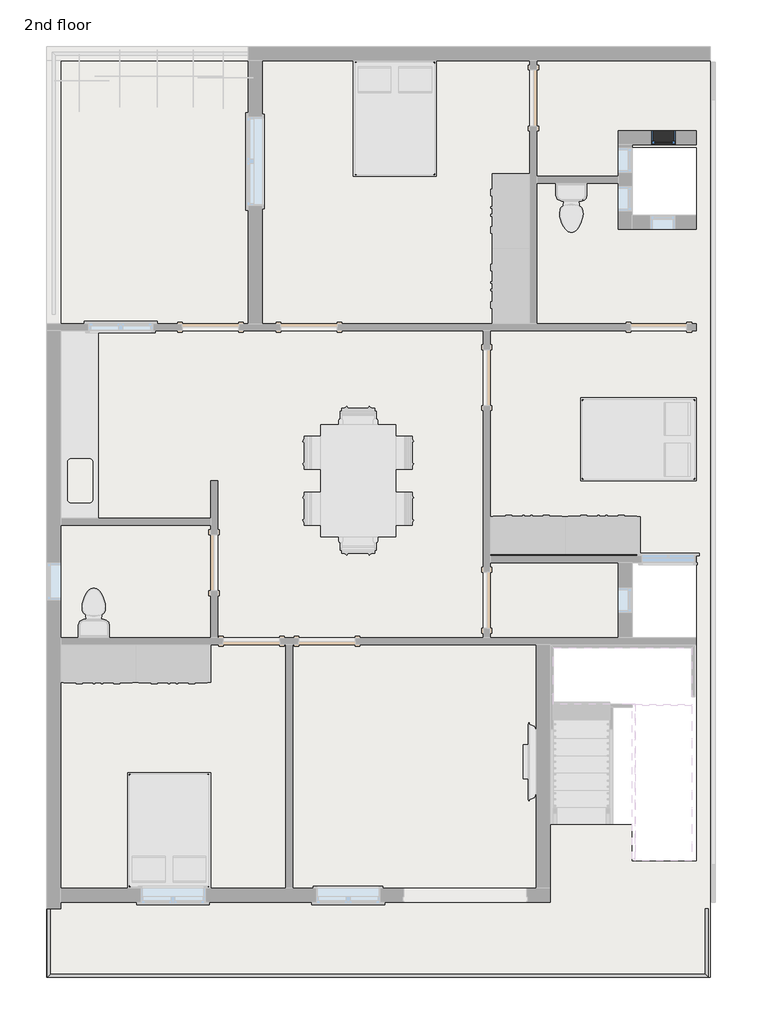
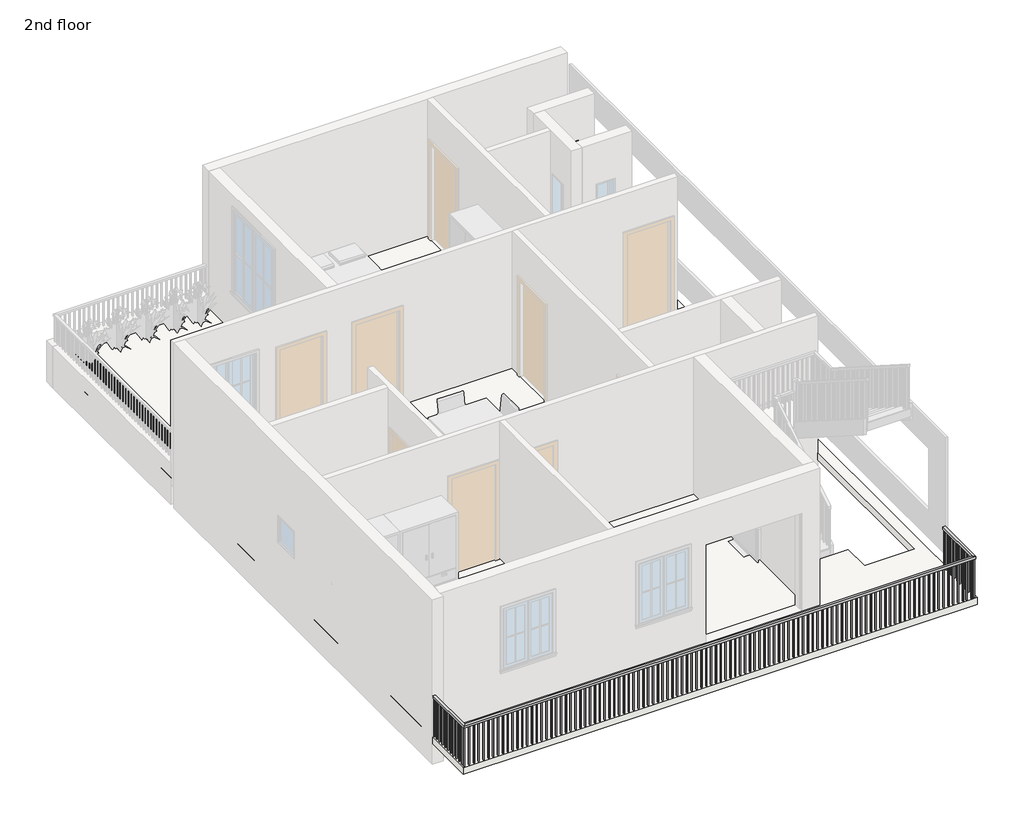
# One storey, part 2 of 5: 1 railing, 1 slab, 1 wall, 1 window.
"""IFC4 building model written with IfcOpenShell, lengths in millimetres."""

from ifc_helpers import new_model, si_unit, frame, origin, place, context, project, spatial, polyline, outline, extrude, faceted_brep, transform, mapped, element, save
from components import window_cea7027f

model = new_model("IFC4")

# Units and contexts
model_context = context("Model", 3, world=origin())
ifc_project = project(units=[si_unit("LENGTHUNIT", "METRE", prefix="MILLI")], contexts=[model_context])

# Site, building, storey
site = spatial("IfcSite", under=ifc_project)
building = spatial("IfcBuilding", under=site)
storey = spatial("IfcBuildingStorey", under=building, Name="2nd floor", Elevation=7010.4)

# Railing
placement = place(None, origin())
element("IfcRailing", 1, ObjectType="Handrail - Rectangular", at=placement, inside=storey, context=model_context, shape_type="SolidModel", body=[
    faceted_brep([(-8046.8498597, -1213.9742075, 7924.8), (-8046.8498597, -1213.9742075, 7874.0), (-8097.6498597, -1213.9742075, 7874.0), (-8097.6498597, -1213.9742075, 7924.8), (-8046.8498597, -2280.7742075, 7924.8), (-8046.8498597, -2280.7742075, 7874.0), (-8097.6498597, -2331.5742075, 7874.0), (-8097.6498597, -2331.5742075, 7924.8), (2602.1001403, -2280.7742075, 7924.8), (2602.1001403, -2280.7742075, 7874.0), (2652.9001403, -2331.5742075, 7874.0), (2652.9001403, -2331.5742075, 7924.8), (2602.1001403, -1213.9742075, 7924.8), (2652.9001403, -1213.9742075, 7924.8), (2652.9001403, -1213.9742075, 7874.0), (2602.1001403, -1213.9742075, 7874.0)], [[[0, 1, 2, 3]], [[1, 0, 4, 5]], [[2, 1, 5, 6]], [[3, 2, 6, 7]], [[0, 3, 7, 4]], [[5, 4, 8, 9]], [[6, 5, 9, 10]], [[7, 6, 10, 11]], [[4, 7, 11, 8]], [[12, 13, 14, 15]], [[9, 8, 12, 15]], [[10, 9, 15, 14]], [[11, 10, 14, 13]], [[8, 11, 13, 12]]]),
    extrude(outline(polyline([(2637.0251403, -1299.6992075), (2617.9751403, -1299.6992075), (2617.9751403, -1280.6492075), (2637.0251403, -1280.6492075), (2637.0251403, -1299.6992075)])), frame((0.0, 0.0, 7010.4), z_axis=(0.0, 0.0, 1.0), x_axis=(1.0, 0.0, 0.0)), (0.0, 0.0, 1.0), 863.6),
    extrude(outline(polyline([(2637.0251403, -1401.2992075), (2617.9751403, -1401.2992075), (2617.9751403, -1382.2492075), (2637.0251403, -1382.2492075), (2637.0251403, -1401.2992075)])), frame((0.0, 0.0, 7010.4), z_axis=(0.0, 0.0, 1.0), x_axis=(1.0, 0.0, 0.0)), (0.0, 0.0, 1.0), 863.6),
    extrude(outline(polyline([(2637.0251403, -1502.8992075), (2617.9751403, -1502.8992075), (2617.9751403, -1483.8492075), (2637.0251403, -1483.8492075), (2637.0251403, -1502.8992075)])), frame((0.0, 0.0, 7010.4), z_axis=(0.0, 0.0, 1.0), x_axis=(1.0, 0.0, 0.0)), (0.0, 0.0, 1.0), 863.6),
    extrude(outline(polyline([(2637.0251403, -1604.4992075), (2617.9751403, -1604.4992075), (2617.9751403, -1585.4492075), (2637.0251403, -1585.4492075), (2637.0251403, -1604.4992075)])), frame((0.0, 0.0, 7010.4), z_axis=(0.0, 0.0, 1.0), x_axis=(1.0, 0.0, 0.0)), (0.0, 0.0, 1.0), 863.6),
    extrude(outline(polyline([(2637.0251403, -1706.0992075), (2617.9751403, -1706.0992075), (2617.9751403, -1687.0492075), (2637.0251403, -1687.0492075), (2637.0251403, -1706.0992075)])), frame((0.0, 0.0, 7010.4), z_axis=(0.0, 0.0, 1.0), x_axis=(1.0, 0.0, 0.0)), (0.0, 0.0, 1.0), 863.6),
    extrude(outline(polyline([(2637.0251403, -1807.6992075), (2617.9751403, -1807.6992075), (2617.9751403, -1788.6492075), (2637.0251403, -1788.6492075), (2637.0251403, -1807.6992075)])), frame((0.0, 0.0, 7010.4), z_axis=(0.0, 0.0, 1.0), x_axis=(1.0, 0.0, 0.0)), (0.0, 0.0, 1.0), 863.6),
    extrude(outline(polyline([(2637.0251403, -1909.2992075), (2617.9751403, -1909.2992075), (2617.9751403, -1890.2492075), (2637.0251403, -1890.2492075), (2637.0251403, -1909.2992075)])), frame((0.0, 0.0, 7010.4), z_axis=(0.0, 0.0, 1.0), x_axis=(1.0, 0.0, 0.0)), (0.0, 0.0, 1.0), 863.6),
    extrude(outline(polyline([(2637.0251403, -2010.8992075), (2617.9751403, -2010.8992075), (2617.9751403, -1991.8492075), (2637.0251403, -1991.8492075), (2637.0251403, -2010.8992075)])), frame((0.0, 0.0, 7010.4), z_axis=(0.0, 0.0, 1.0), x_axis=(1.0, 0.0, 0.0)), (0.0, 0.0, 1.0), 863.6),
    extrude(outline(polyline([(2637.0251403, -2112.4992075), (2617.9751403, -2112.4992075), (2617.9751403, -2093.4492075), (2637.0251403, -2093.4492075), (2637.0251403, -2112.4992075)])), frame((0.0, 0.0, 7010.4), z_axis=(0.0, 0.0, 1.0), x_axis=(1.0, 0.0, 0.0)), (0.0, 0.0, 1.0), 863.6),
    extrude(outline(polyline([(2637.0251403, -2214.0992075), (2617.9751403, -2214.0992075), (2617.9751403, -2195.0492075), (2637.0251403, -2195.0492075), (2637.0251403, -2214.0992075)])), frame((0.0, 0.0, 7010.4), z_axis=(0.0, 0.0, 1.0), x_axis=(1.0, 0.0, 0.0)), (0.0, 0.0, 1.0), 863.6),
    extrude(outline(polyline([(2560.8251403, -2315.6992075), (2560.8251403, -2296.6492075), (2579.8751403, -2296.6492075), (2579.8751403, -2315.6992075), (2560.8251403, -2315.6992075)])), frame((0.0, 0.0, 7010.4), z_axis=(0.0, 0.0, 1.0), x_axis=(1.0, 0.0, 0.0)), (0.0, 0.0, 1.0), 863.6),
    extrude(outline(polyline([(2383.0251403, -2315.6992075), (2383.0251403, -2296.6492075), (2402.0751403, -2296.6492075), (2402.0751403, -2315.6992075), (2383.0251403, -2315.6992075)])), frame((0.0, 0.0, 7010.4), z_axis=(0.0, 0.0, 1.0), x_axis=(1.0, 0.0, 0.0)), (0.0, 0.0, 1.0), 863.6),
    extrude(outline(polyline([(2281.4251403, -2315.6992075), (2281.4251403, -2296.6492075), (2300.4751403, -2296.6492075), (2300.4751403, -2315.6992075), (2281.4251403, -2315.6992075)])), frame((0.0, 0.0, 7010.4), z_axis=(0.0, 0.0, 1.0), x_axis=(1.0, 0.0, 0.0)), (0.0, 0.0, 1.0), 863.6),
    extrude(outline(polyline([(2179.8251403, -2315.6992075), (2179.8251403, -2296.6492075), (2198.8751403, -2296.6492075), (2198.8751403, -2315.6992075), (2179.8251403, -2315.6992075)])), frame((0.0, 0.0, 7010.4), z_axis=(0.0, 0.0, 1.0), x_axis=(1.0, 0.0, 0.0)), (0.0, 0.0, 1.0), 863.6),
    extrude(outline(polyline([(2078.2251403, -2315.6992075), (2078.2251403, -2296.6492075), (2097.2751403, -2296.6492075), (2097.2751403, -2315.6992075), (2078.2251403, -2315.6992075)])), frame((0.0, 0.0, 7010.4), z_axis=(0.0, 0.0, 1.0), x_axis=(1.0, 0.0, 0.0)), (0.0, 0.0, 1.0), 863.6),
    extrude(outline(polyline([(1976.6251403, -2315.6992075), (1976.6251403, -2296.6492075), (1995.6751403, -2296.6492075), (1995.6751403, -2315.6992075), (1976.6251403, -2315.6992075)])), frame((0.0, 0.0, 7010.4), z_axis=(0.0, 0.0, 1.0), x_axis=(1.0, 0.0, 0.0)), (0.0, 0.0, 1.0), 863.6),
    extrude(outline(polyline([(1875.0251403, -2315.6992075), (1875.0251403, -2296.6492075), (1894.0751403, -2296.6492075), (1894.0751403, -2315.6992075), (1875.0251403, -2315.6992075)])), frame((0.0, 0.0, 7010.4), z_axis=(0.0, 0.0, 1.0), x_axis=(1.0, 0.0, 0.0)), (0.0, 0.0, 1.0), 863.6),
    extrude(outline(polyline([(1773.4251403, -2315.6992075), (1773.4251403, -2296.6492075), (1792.4751403, -2296.6492075), (1792.4751403, -2315.6992075), (1773.4251403, -2315.6992075)])), frame((0.0, 0.0, 7010.4), z_axis=(0.0, 0.0, 1.0), x_axis=(1.0, 0.0, 0.0)), (0.0, 0.0, 1.0), 863.6),
    extrude(outline(polyline([(1671.8251403, -2315.6992075), (1671.8251403, -2296.6492075), (1690.8751403, -2296.6492075), (1690.8751403, -2315.6992075), (1671.8251403, -2315.6992075)])), frame((0.0, 0.0, 7010.4), z_axis=(0.0, 0.0, 1.0), x_axis=(1.0, 0.0, 0.0)), (0.0, 0.0, 1.0), 863.6),
    extrude(outline(polyline([(1570.2251403, -2315.6992075), (1570.2251403, -2296.6492075), (1589.2751403, -2296.6492075), (1589.2751403, -2315.6992075), (1570.2251403, -2315.6992075)])), frame((0.0, 0.0, 7010.4), z_axis=(0.0, 0.0, 1.0), x_axis=(1.0, 0.0, 0.0)), (0.0, 0.0, 1.0), 863.6),
    extrude(outline(polyline([(1468.6251403, -2315.6992075), (1468.6251403, -2296.6492075), (1487.6751403, -2296.6492075), (1487.6751403, -2315.6992075), (1468.6251403, -2315.6992075)])), frame((0.0, 0.0, 7010.4), z_axis=(0.0, 0.0, 1.0), x_axis=(1.0, 0.0, 0.0)), (0.0, 0.0, 1.0), 863.6),
    extrude(outline(polyline([(1367.0251403, -2315.6992075), (1367.0251403, -2296.6492075), (1386.0751403, -2296.6492075), (1386.0751403, -2315.6992075), (1367.0251403, -2315.6992075)])), frame((0.0, 0.0, 7010.4), z_axis=(0.0, 0.0, 1.0), x_axis=(1.0, 0.0, 0.0)), (0.0, 0.0, 1.0), 863.6),
    extrude(outline(polyline([(1265.4251403, -2315.6992075), (1265.4251403, -2296.6492075), (1284.4751403, -2296.6492075), (1284.4751403, -2315.6992075), (1265.4251403, -2315.6992075)])), frame((0.0, 0.0, 7010.4), z_axis=(0.0, 0.0, 1.0), x_axis=(1.0, 0.0, 0.0)), (0.0, 0.0, 1.0), 863.6),
    extrude(outline(polyline([(1163.8251403, -2315.6992075), (1163.8251403, -2296.6492075), (1182.8751403, -2296.6492075), (1182.8751403, -2315.6992075), (1163.8251403, -2315.6992075)])), frame((0.0, 0.0, 7010.4), z_axis=(0.0, 0.0, 1.0), x_axis=(1.0, 0.0, 0.0)), (0.0, 0.0, 1.0), 863.6),
    extrude(outline(polyline([(1062.2251403, -2315.6992075), (1062.2251403, -2296.6492075), (1081.2751403, -2296.6492075), (1081.2751403, -2315.6992075), (1062.2251403, -2315.6992075)])), frame((0.0, 0.0, 7010.4), z_axis=(0.0, 0.0, 1.0), x_axis=(1.0, 0.0, 0.0)), (0.0, 0.0, 1.0), 863.6),
    extrude(outline(polyline([(960.6251403, -2315.6992075), (960.6251403, -2296.6492075), (979.6751403, -2296.6492075), (979.6751403, -2315.6992075), (960.6251403, -2315.6992075)])), frame((0.0, 0.0, 7010.4), z_axis=(0.0, 0.0, 1.0), x_axis=(1.0, 0.0, 0.0)), (0.0, 0.0, 1.0), 863.6),
    extrude(outline(polyline([(859.0251403, -2315.6992075), (859.0251403, -2296.6492075), (878.0751403, -2296.6492075), (878.0751403, -2315.6992075), (859.0251403, -2315.6992075)])), frame((0.0, 0.0, 7010.4), z_axis=(0.0, 0.0, 1.0), x_axis=(1.0, 0.0, 0.0)), (0.0, 0.0, 1.0), 863.6),
    extrude(outline(polyline([(757.4251403, -2315.6992075), (757.4251403, -2296.6492075), (776.4751403, -2296.6492075), (776.4751403, -2315.6992075), (757.4251403, -2315.6992075)])), frame((0.0, 0.0, 7010.4), z_axis=(0.0, 0.0, 1.0), x_axis=(1.0, 0.0, 0.0)), (0.0, 0.0, 1.0), 863.6),
    extrude(outline(polyline([(655.8251403, -2315.6992075), (655.8251403, -2296.6492075), (674.8751403, -2296.6492075), (674.8751403, -2315.6992075), (655.8251403, -2315.6992075)])), frame((0.0, 0.0, 7010.4), z_axis=(0.0, 0.0, 1.0), x_axis=(1.0, 0.0, 0.0)), (0.0, 0.0, 1.0), 863.6),
    extrude(outline(polyline([(554.2251403, -2315.6992075), (554.2251403, -2296.6492075), (573.2751403, -2296.6492075), (573.2751403, -2315.6992075), (554.2251403, -2315.6992075)])), frame((0.0, 0.0, 7010.4), z_axis=(0.0, 0.0, 1.0), x_axis=(1.0, 0.0, 0.0)), (0.0, 0.0, 1.0), 863.6),
    extrude(outline(polyline([(452.6251403, -2315.6992075), (452.6251403, -2296.6492075), (471.6751403, -2296.6492075), (471.6751403, -2315.6992075), (452.6251403, -2315.6992075)])), frame((0.0, 0.0, 7010.4), z_axis=(0.0, 0.0, 1.0), x_axis=(1.0, 0.0, 0.0)), (0.0, 0.0, 1.0), 863.6),
    extrude(outline(polyline([(351.0251403, -2315.6992075), (351.0251403, -2296.6492075), (370.0751403, -2296.6492075), (370.0751403, -2315.6992075), (351.0251403, -2315.6992075)])), frame((0.0, 0.0, 7010.4), z_axis=(0.0, 0.0, 1.0), x_axis=(1.0, 0.0, 0.0)), (0.0, 0.0, 1.0), 863.6),
    extrude(outline(polyline([(249.4251403, -2315.6992075), (249.4251403, -2296.6492075), (268.4751403, -2296.6492075), (268.4751403, -2315.6992075), (249.4251403, -2315.6992075)])), frame((0.0, 0.0, 7010.4), z_axis=(0.0, 0.0, 1.0), x_axis=(1.0, 0.0, 0.0)), (0.0, 0.0, 1.0), 863.6),
    extrude(outline(polyline([(147.8251403, -2315.6992075), (147.8251403, -2296.6492075), (166.8751403, -2296.6492075), (166.8751403, -2315.6992075), (147.8251403, -2315.6992075)])), frame((0.0, 0.0, 7010.4), z_axis=(0.0, 0.0, 1.0), x_axis=(1.0, 0.0, 0.0)), (0.0, 0.0, 1.0), 863.6),
    extrude(outline(polyline([(46.2251403, -2315.6992075), (46.2251403, -2296.6492075), (65.2751403, -2296.6492075), (65.2751403, -2315.6992075), (46.2251403, -2315.6992075)])), frame((0.0, 0.0, 7010.4), z_axis=(0.0, 0.0, 1.0), x_axis=(1.0, 0.0, 0.0)), (0.0, 0.0, 1.0), 863.6),
    extrude(outline(polyline([(-55.3748597, -2315.6992075), (-55.3748597, -2296.6492075), (-36.3248597, -2296.6492075), (-36.3248597, -2315.6992075), (-55.3748597, -2315.6992075)])), frame((0.0, 0.0, 7010.4), z_axis=(0.0, 0.0, 1.0), x_axis=(1.0, 0.0, 0.0)), (0.0, 0.0, 1.0), 863.6),
    extrude(outline(polyline([(-156.9748597, -2315.6992075), (-156.9748597, -2296.6492075), (-137.9248597, -2296.6492075), (-137.9248597, -2315.6992075), (-156.9748597, -2315.6992075)])), frame((0.0, 0.0, 7010.4), z_axis=(0.0, 0.0, 1.0), x_axis=(1.0, 0.0, 0.0)), (0.0, 0.0, 1.0), 863.6),
    extrude(outline(polyline([(-258.5748597, -2315.6992075), (-258.5748597, -2296.6492075), (-239.5248597, -2296.6492075), (-239.5248597, -2315.6992075), (-258.5748597, -2315.6992075)])), frame((0.0, 0.0, 7010.4), z_axis=(0.0, 0.0, 1.0), x_axis=(1.0, 0.0, 0.0)), (0.0, 0.0, 1.0), 863.6),
    extrude(outline(polyline([(-360.1748597, -2315.6992075), (-360.1748597, -2296.6492075), (-341.1248597, -2296.6492075), (-341.1248597, -2315.6992075), (-360.1748597, -2315.6992075)])), frame((0.0, 0.0, 7010.4), z_axis=(0.0, 0.0, 1.0), x_axis=(1.0, 0.0, 0.0)), (0.0, 0.0, 1.0), 863.6),
    extrude(outline(polyline([(-461.7748597, -2315.6992075), (-461.7748597, -2296.6492075), (-442.7248597, -2296.6492075), (-442.7248597, -2315.6992075), (-461.7748597, -2315.6992075)])), frame((0.0, 0.0, 7010.4), z_axis=(0.0, 0.0, 1.0), x_axis=(1.0, 0.0, 0.0)), (0.0, 0.0, 1.0), 863.6),
    extrude(outline(polyline([(-563.3748597, -2315.6992075), (-563.3748597, -2296.6492075), (-544.3248597, -2296.6492075), (-544.3248597, -2315.6992075), (-563.3748597, -2315.6992075)])), frame((0.0, 0.0, 7010.4), z_axis=(0.0, 0.0, 1.0), x_axis=(1.0, 0.0, 0.0)), (0.0, 0.0, 1.0), 863.6),
    extrude(outline(polyline([(-664.9748597, -2315.6992075), (-664.9748597, -2296.6492075), (-645.9248597, -2296.6492075), (-645.9248597, -2315.6992075), (-664.9748597, -2315.6992075)])), frame((0.0, 0.0, 7010.4), z_axis=(0.0, 0.0, 1.0), x_axis=(1.0, 0.0, 0.0)), (0.0, 0.0, 1.0), 863.6),
    extrude(outline(polyline([(-766.5748597, -2315.6992075), (-766.5748597, -2296.6492075), (-747.5248597, -2296.6492075), (-747.5248597, -2315.6992075), (-766.5748597, -2315.6992075)])), frame((0.0, 0.0, 7010.4), z_axis=(0.0, 0.0, 1.0), x_axis=(1.0, 0.0, 0.0)), (0.0, 0.0, 1.0), 863.6),
    extrude(outline(polyline([(-868.1748597, -2315.6992075), (-868.1748597, -2296.6492075), (-849.1248597, -2296.6492075), (-849.1248597, -2315.6992075), (-868.1748597, -2315.6992075)])), frame((0.0, 0.0, 7010.4), z_axis=(0.0, 0.0, 1.0), x_axis=(1.0, 0.0, 0.0)), (0.0, 0.0, 1.0), 863.6),
    extrude(outline(polyline([(-969.7748597, -2315.6992075), (-969.7748597, -2296.6492075), (-950.7248597, -2296.6492075), (-950.7248597, -2315.6992075), (-969.7748597, -2315.6992075)])), frame((0.0, 0.0, 7010.4), z_axis=(0.0, 0.0, 1.0), x_axis=(1.0, 0.0, 0.0)), (0.0, 0.0, 1.0), 863.6),
    extrude(outline(polyline([(-1071.3748597, -2315.6992075), (-1071.3748597, -2296.6492075), (-1052.3248597, -2296.6492075), (-1052.3248597, -2315.6992075), (-1071.3748597, -2315.6992075)])), frame((0.0, 0.0, 7010.4), z_axis=(0.0, 0.0, 1.0), x_axis=(1.0, 0.0, 0.0)), (0.0, 0.0, 1.0), 863.6),
    extrude(outline(polyline([(-1172.9748597, -2315.6992075), (-1172.9748597, -2296.6492075), (-1153.9248597, -2296.6492075), (-1153.9248597, -2315.6992075), (-1172.9748597, -2315.6992075)])), frame((0.0, 0.0, 7010.4), z_axis=(0.0, 0.0, 1.0), x_axis=(1.0, 0.0, 0.0)), (0.0, 0.0, 1.0), 863.6),
    extrude(outline(polyline([(-1274.5748597, -2315.6992075), (-1274.5748597, -2296.6492075), (-1255.5248597, -2296.6492075), (-1255.5248597, -2315.6992075), (-1274.5748597, -2315.6992075)])), frame((0.0, 0.0, 7010.4), z_axis=(0.0, 0.0, 1.0), x_axis=(1.0, 0.0, 0.0)), (0.0, 0.0, 1.0), 863.6),
    extrude(outline(polyline([(-1376.1748597, -2315.6992075), (-1376.1748597, -2296.6492075), (-1357.1248597, -2296.6492075), (-1357.1248597, -2315.6992075), (-1376.1748597, -2315.6992075)])), frame((0.0, 0.0, 7010.4), z_axis=(0.0, 0.0, 1.0), x_axis=(1.0, 0.0, 0.0)), (0.0, 0.0, 1.0), 863.6),
    extrude(outline(polyline([(-1477.7748597, -2315.6992075), (-1477.7748597, -2296.6492075), (-1458.7248597, -2296.6492075), (-1458.7248597, -2315.6992075), (-1477.7748597, -2315.6992075)])), frame((0.0, 0.0, 7010.4), z_axis=(0.0, 0.0, 1.0), x_axis=(1.0, 0.0, 0.0)), (0.0, 0.0, 1.0), 863.6),
    extrude(outline(polyline([(-1579.3748597, -2315.6992075), (-1579.3748597, -2296.6492075), (-1560.3248597, -2296.6492075), (-1560.3248597, -2315.6992075), (-1579.3748597, -2315.6992075)])), frame((0.0, 0.0, 7010.4), z_axis=(0.0, 0.0, 1.0), x_axis=(1.0, 0.0, 0.0)), (0.0, 0.0, 1.0), 863.6),
    extrude(outline(polyline([(-1680.9748597, -2315.6992075), (-1680.9748597, -2296.6492075), (-1661.9248597, -2296.6492075), (-1661.9248597, -2315.6992075), (-1680.9748597, -2315.6992075)])), frame((0.0, 0.0, 7010.4), z_axis=(0.0, 0.0, 1.0), x_axis=(1.0, 0.0, 0.0)), (0.0, 0.0, 1.0), 863.6),
    extrude(outline(polyline([(-1782.5748597, -2315.6992075), (-1782.5748597, -2296.6492075), (-1763.5248597, -2296.6492075), (-1763.5248597, -2315.6992075), (-1782.5748597, -2315.6992075)])), frame((0.0, 0.0, 7010.4), z_axis=(0.0, 0.0, 1.0), x_axis=(1.0, 0.0, 0.0)), (0.0, 0.0, 1.0), 863.6),
    extrude(outline(polyline([(-1884.1748597, -2315.6992075), (-1884.1748597, -2296.6492075), (-1865.1248597, -2296.6492075), (-1865.1248597, -2315.6992075), (-1884.1748597, -2315.6992075)])), frame((0.0, 0.0, 7010.4), z_axis=(0.0, 0.0, 1.0), x_axis=(1.0, 0.0, 0.0)), (0.0, 0.0, 1.0), 863.6),
    extrude(outline(polyline([(-1985.7748597, -2315.6992075), (-1985.7748597, -2296.6492075), (-1966.7248597, -2296.6492075), (-1966.7248597, -2315.6992075), (-1985.7748597, -2315.6992075)])), frame((0.0, 0.0, 7010.4), z_axis=(0.0, 0.0, 1.0), x_axis=(1.0, 0.0, 0.0)), (0.0, 0.0, 1.0), 863.6),
    extrude(outline(polyline([(-2087.3748597, -2315.6992075), (-2087.3748597, -2296.6492075), (-2068.3248597, -2296.6492075), (-2068.3248597, -2315.6992075), (-2087.3748597, -2315.6992075)])), frame((0.0, 0.0, 7010.4), z_axis=(0.0, 0.0, 1.0), x_axis=(1.0, 0.0, 0.0)), (0.0, 0.0, 1.0), 863.6),
    extrude(outline(polyline([(-2188.9748597, -2315.6992075), (-2188.9748597, -2296.6492075), (-2169.9248597, -2296.6492075), (-2169.9248597, -2315.6992075), (-2188.9748597, -2315.6992075)])), frame((0.0, 0.0, 7010.4), z_axis=(0.0, 0.0, 1.0), x_axis=(1.0, 0.0, 0.0)), (0.0, 0.0, 1.0), 863.6),
    extrude(outline(polyline([(-2290.5748597, -2315.6992075), (-2290.5748597, -2296.6492075), (-2271.5248597, -2296.6492075), (-2271.5248597, -2315.6992075), (-2290.5748597, -2315.6992075)])), frame((0.0, 0.0, 7010.4), z_axis=(0.0, 0.0, 1.0), x_axis=(1.0, 0.0, 0.0)), (0.0, 0.0, 1.0), 863.6),
    extrude(outline(polyline([(-2392.1748597, -2315.6992075), (-2392.1748597, -2296.6492075), (-2373.1248597, -2296.6492075), (-2373.1248597, -2315.6992075), (-2392.1748597, -2315.6992075)])), frame((0.0, 0.0, 7010.4), z_axis=(0.0, 0.0, 1.0), x_axis=(1.0, 0.0, 0.0)), (0.0, 0.0, 1.0), 863.6),
    extrude(outline(polyline([(-2493.7748597, -2315.6992075), (-2493.7748597, -2296.6492075), (-2474.7248597, -2296.6492075), (-2474.7248597, -2315.6992075), (-2493.7748597, -2315.6992075)])), frame((0.0, 0.0, 7010.4), z_axis=(0.0, 0.0, 1.0), x_axis=(1.0, 0.0, 0.0)), (0.0, 0.0, 1.0), 863.6),
    extrude(outline(polyline([(-2595.3748597, -2315.6992075), (-2595.3748597, -2296.6492075), (-2576.3248597, -2296.6492075), (-2576.3248597, -2315.6992075), (-2595.3748597, -2315.6992075)])), frame((0.0, 0.0, 7010.4), z_axis=(0.0, 0.0, 1.0), x_axis=(1.0, 0.0, 0.0)), (0.0, 0.0, 1.0), 863.6),
    extrude(outline(polyline([(-2696.9748597, -2315.6992075), (-2696.9748597, -2296.6492075), (-2677.9248597, -2296.6492075), (-2677.9248597, -2315.6992075), (-2696.9748597, -2315.6992075)])), frame((0.0, 0.0, 7010.4), z_axis=(0.0, 0.0, 1.0), x_axis=(1.0, 0.0, 0.0)), (0.0, 0.0, 1.0), 863.6),
    extrude(outline(polyline([(-2798.5748597, -2315.6992075), (-2798.5748597, -2296.6492075), (-2779.5248597, -2296.6492075), (-2779.5248597, -2315.6992075), (-2798.5748597, -2315.6992075)])), frame((0.0, 0.0, 7010.4), z_axis=(0.0, 0.0, 1.0), x_axis=(1.0, 0.0, 0.0)), (0.0, 0.0, 1.0), 863.6),
    extrude(outline(polyline([(-2900.1748597, -2315.6992075), (-2900.1748597, -2296.6492075), (-2881.1248597, -2296.6492075), (-2881.1248597, -2315.6992075), (-2900.1748597, -2315.6992075)])), frame((0.0, 0.0, 7010.4), z_axis=(0.0, 0.0, 1.0), x_axis=(1.0, 0.0, 0.0)), (0.0, 0.0, 1.0), 863.6),
    extrude(outline(polyline([(-3001.7748597, -2315.6992075), (-3001.7748597, -2296.6492075), (-2982.7248597, -2296.6492075), (-2982.7248597, -2315.6992075), (-3001.7748597, -2315.6992075)])), frame((0.0, 0.0, 7010.4), z_axis=(0.0, 0.0, 1.0), x_axis=(1.0, 0.0, 0.0)), (0.0, 0.0, 1.0), 863.6),
    extrude(outline(polyline([(-3103.3748597, -2315.6992075), (-3103.3748597, -2296.6492075), (-3084.3248597, -2296.6492075), (-3084.3248597, -2315.6992075), (-3103.3748597, -2315.6992075)])), frame((0.0, 0.0, 7010.4), z_axis=(0.0, 0.0, 1.0), x_axis=(1.0, 0.0, 0.0)), (0.0, 0.0, 1.0), 863.6),
    extrude(outline(polyline([(-3204.9748597, -2315.6992075), (-3204.9748597, -2296.6492075), (-3185.9248597, -2296.6492075), (-3185.9248597, -2315.6992075), (-3204.9748597, -2315.6992075)])), frame((0.0, 0.0, 7010.4), z_axis=(0.0, 0.0, 1.0), x_axis=(1.0, 0.0, 0.0)), (0.0, 0.0, 1.0), 863.6),
    extrude(outline(polyline([(-3306.5748597, -2315.6992075), (-3306.5748597, -2296.6492075), (-3287.5248597, -2296.6492075), (-3287.5248597, -2315.6992075), (-3306.5748597, -2315.6992075)])), frame((0.0, 0.0, 7010.4), z_axis=(0.0, 0.0, 1.0), x_axis=(1.0, 0.0, 0.0)), (0.0, 0.0, 1.0), 863.6),
    extrude(outline(polyline([(-3408.1748597, -2315.6992075), (-3408.1748597, -2296.6492075), (-3389.1248597, -2296.6492075), (-3389.1248597, -2315.6992075), (-3408.1748597, -2315.6992075)])), frame((0.0, 0.0, 7010.4), z_axis=(0.0, 0.0, 1.0), x_axis=(1.0, 0.0, 0.0)), (0.0, 0.0, 1.0), 863.6),
    extrude(outline(polyline([(-3509.7748597, -2315.6992075), (-3509.7748597, -2296.6492075), (-3490.7248597, -2296.6492075), (-3490.7248597, -2315.6992075), (-3509.7748597, -2315.6992075)])), frame((0.0, 0.0, 7010.4), z_axis=(0.0, 0.0, 1.0), x_axis=(1.0, 0.0, 0.0)), (0.0, 0.0, 1.0), 863.6),
    extrude(outline(polyline([(-3611.3748597, -2315.6992075), (-3611.3748597, -2296.6492075), (-3592.3248597, -2296.6492075), (-3592.3248597, -2315.6992075), (-3611.3748597, -2315.6992075)])), frame((0.0, 0.0, 7010.4), z_axis=(0.0, 0.0, 1.0), x_axis=(1.0, 0.0, 0.0)), (0.0, 0.0, 1.0), 863.6),
    extrude(outline(polyline([(-3712.9748597, -2315.6992075), (-3712.9748597, -2296.6492075), (-3693.9248597, -2296.6492075), (-3693.9248597, -2315.6992075), (-3712.9748597, -2315.6992075)])), frame((0.0, 0.0, 7010.4), z_axis=(0.0, 0.0, 1.0), x_axis=(1.0, 0.0, 0.0)), (0.0, 0.0, 1.0), 863.6),
    extrude(outline(polyline([(-3814.5748597, -2315.6992075), (-3814.5748597, -2296.6492075), (-3795.5248597, -2296.6492075), (-3795.5248597, -2315.6992075), (-3814.5748597, -2315.6992075)])), frame((0.0, 0.0, 7010.4), z_axis=(0.0, 0.0, 1.0), x_axis=(1.0, 0.0, 0.0)), (0.0, 0.0, 1.0), 863.6),
    extrude(outline(polyline([(-3916.1748597, -2315.6992075), (-3916.1748597, -2296.6492075), (-3897.1248597, -2296.6492075), (-3897.1248597, -2315.6992075), (-3916.1748597, -2315.6992075)])), frame((0.0, 0.0, 7010.4), z_axis=(0.0, 0.0, 1.0), x_axis=(1.0, 0.0, 0.0)), (0.0, 0.0, 1.0), 863.6),
    extrude(outline(polyline([(-4017.7748597, -2315.6992075), (-4017.7748597, -2296.6492075), (-3998.7248597, -2296.6492075), (-3998.7248597, -2315.6992075), (-4017.7748597, -2315.6992075)])), frame((0.0, 0.0, 7010.4), z_axis=(0.0, 0.0, 1.0), x_axis=(1.0, 0.0, 0.0)), (0.0, 0.0, 1.0), 863.6),
    extrude(outline(polyline([(-4119.3748597, -2315.6992075), (-4119.3748597, -2296.6492075), (-4100.3248597, -2296.6492075), (-4100.3248597, -2315.6992075), (-4119.3748597, -2315.6992075)])), frame((0.0, 0.0, 7010.4), z_axis=(0.0, 0.0, 1.0), x_axis=(1.0, 0.0, 0.0)), (0.0, 0.0, 1.0), 863.6),
    extrude(outline(polyline([(-4220.9748597, -2315.6992075), (-4220.9748597, -2296.6492075), (-4201.9248597, -2296.6492075), (-4201.9248597, -2315.6992075), (-4220.9748597, -2315.6992075)])), frame((0.0, 0.0, 7010.4), z_axis=(0.0, 0.0, 1.0), x_axis=(1.0, 0.0, 0.0)), (0.0, 0.0, 1.0), 863.6),
    extrude(outline(polyline([(-4322.5748597, -2315.6992075), (-4322.5748597, -2296.6492075), (-4303.5248597, -2296.6492075), (-4303.5248597, -2315.6992075), (-4322.5748597, -2315.6992075)])), frame((0.0, 0.0, 7010.4), z_axis=(0.0, 0.0, 1.0), x_axis=(1.0, 0.0, 0.0)), (0.0, 0.0, 1.0), 863.6),
    extrude(outline(polyline([(-4424.1748597, -2315.6992075), (-4424.1748597, -2296.6492075), (-4405.1248597, -2296.6492075), (-4405.1248597, -2315.6992075), (-4424.1748597, -2315.6992075)])), frame((0.0, 0.0, 7010.4), z_axis=(0.0, 0.0, 1.0), x_axis=(1.0, 0.0, 0.0)), (0.0, 0.0, 1.0), 863.6),
    extrude(outline(polyline([(-4525.7748597, -2315.6992075), (-4525.7748597, -2296.6492075), (-4506.7248597, -2296.6492075), (-4506.7248597, -2315.6992075), (-4525.7748597, -2315.6992075)])), frame((0.0, 0.0, 7010.4), z_axis=(0.0, 0.0, 1.0), x_axis=(1.0, 0.0, 0.0)), (0.0, 0.0, 1.0), 863.6),
    extrude(outline(polyline([(-4627.3748597, -2315.6992075), (-4627.3748597, -2296.6492075), (-4608.3248597, -2296.6492075), (-4608.3248597, -2315.6992075), (-4627.3748597, -2315.6992075)])), frame((0.0, 0.0, 7010.4), z_axis=(0.0, 0.0, 1.0), x_axis=(1.0, 0.0, 0.0)), (0.0, 0.0, 1.0), 863.6),
    extrude(outline(polyline([(-4728.9748597, -2315.6992075), (-4728.9748597, -2296.6492075), (-4709.9248597, -2296.6492075), (-4709.9248597, -2315.6992075), (-4728.9748597, -2315.6992075)])), frame((0.0, 0.0, 7010.4), z_axis=(0.0, 0.0, 1.0), x_axis=(1.0, 0.0, 0.0)), (0.0, 0.0, 1.0), 863.6),
    extrude(outline(polyline([(-4830.5748597, -2315.6992075), (-4830.5748597, -2296.6492075), (-4811.5248597, -2296.6492075), (-4811.5248597, -2315.6992075), (-4830.5748597, -2315.6992075)])), frame((0.0, 0.0, 7010.4), z_axis=(0.0, 0.0, 1.0), x_axis=(1.0, 0.0, 0.0)), (0.0, 0.0, 1.0), 863.6),
    extrude(outline(polyline([(-4932.1748597, -2315.6992075), (-4932.1748597, -2296.6492075), (-4913.1248597, -2296.6492075), (-4913.1248597, -2315.6992075), (-4932.1748597, -2315.6992075)])), frame((0.0, 0.0, 7010.4), z_axis=(0.0, 0.0, 1.0), x_axis=(1.0, 0.0, 0.0)), (0.0, 0.0, 1.0), 863.6),
    extrude(outline(polyline([(-5033.7748597, -2315.6992075), (-5033.7748597, -2296.6492075), (-5014.7248597, -2296.6492075), (-5014.7248597, -2315.6992075), (-5033.7748597, -2315.6992075)])), frame((0.0, 0.0, 7010.4), z_axis=(0.0, 0.0, 1.0), x_axis=(1.0, 0.0, 0.0)), (0.0, 0.0, 1.0), 863.6),
    extrude(outline(polyline([(-5135.3748597, -2315.6992075), (-5135.3748597, -2296.6492075), (-5116.3248597, -2296.6492075), (-5116.3248597, -2315.6992075), (-5135.3748597, -2315.6992075)])), frame((0.0, 0.0, 7010.4), z_axis=(0.0, 0.0, 1.0), x_axis=(1.0, 0.0, 0.0)), (0.0, 0.0, 1.0), 863.6),
    extrude(outline(polyline([(-5236.9748597, -2315.6992075), (-5236.9748597, -2296.6492075), (-5217.9248597, -2296.6492075), (-5217.9248597, -2315.6992075), (-5236.9748597, -2315.6992075)])), frame((0.0, 0.0, 7010.4), z_axis=(0.0, 0.0, 1.0), x_axis=(1.0, 0.0, 0.0)), (0.0, 0.0, 1.0), 863.6),
    extrude(outline(polyline([(-5338.5748597, -2315.6992075), (-5338.5748597, -2296.6492075), (-5319.5248597, -2296.6492075), (-5319.5248597, -2315.6992075), (-5338.5748597, -2315.6992075)])), frame((0.0, 0.0, 7010.4), z_axis=(0.0, 0.0, 1.0), x_axis=(1.0, 0.0, 0.0)), (0.0, 0.0, 1.0), 863.6),
    extrude(outline(polyline([(-5440.1748597, -2315.6992075), (-5440.1748597, -2296.6492075), (-5421.1248597, -2296.6492075), (-5421.1248597, -2315.6992075), (-5440.1748597, -2315.6992075)])), frame((0.0, 0.0, 7010.4), z_axis=(0.0, 0.0, 1.0), x_axis=(1.0, 0.0, 0.0)), (0.0, 0.0, 1.0), 863.6),
    extrude(outline(polyline([(-5541.7748597, -2315.6992075), (-5541.7748597, -2296.6492075), (-5522.7248597, -2296.6492075), (-5522.7248597, -2315.6992075), (-5541.7748597, -2315.6992075)])), frame((0.0, 0.0, 7010.4), z_axis=(0.0, 0.0, 1.0), x_axis=(1.0, 0.0, 0.0)), (0.0, 0.0, 1.0), 863.6),
    extrude(outline(polyline([(-5643.3748597, -2315.6992075), (-5643.3748597, -2296.6492075), (-5624.3248597, -2296.6492075), (-5624.3248597, -2315.6992075), (-5643.3748597, -2315.6992075)])), frame((0.0, 0.0, 7010.4), z_axis=(0.0, 0.0, 1.0), x_axis=(1.0, 0.0, 0.0)), (0.0, 0.0, 1.0), 863.6),
    extrude(outline(polyline([(-5744.9748597, -2315.6992075), (-5744.9748597, -2296.6492075), (-5725.9248597, -2296.6492075), (-5725.9248597, -2315.6992075), (-5744.9748597, -2315.6992075)])), frame((0.0, 0.0, 7010.4), z_axis=(0.0, 0.0, 1.0), x_axis=(1.0, 0.0, 0.0)), (0.0, 0.0, 1.0), 863.6),
    extrude(outline(polyline([(-5846.5748597, -2315.6992075), (-5846.5748597, -2296.6492075), (-5827.5248597, -2296.6492075), (-5827.5248597, -2315.6992075), (-5846.5748597, -2315.6992075)])), frame((0.0, 0.0, 7010.4), z_axis=(0.0, 0.0, 1.0), x_axis=(1.0, 0.0, 0.0)), (0.0, 0.0, 1.0), 863.6),
    extrude(outline(polyline([(-5948.1748597, -2315.6992075), (-5948.1748597, -2296.6492075), (-5929.1248597, -2296.6492075), (-5929.1248597, -2315.6992075), (-5948.1748597, -2315.6992075)])), frame((0.0, 0.0, 7010.4), z_axis=(0.0, 0.0, 1.0), x_axis=(1.0, 0.0, 0.0)), (0.0, 0.0, 1.0), 863.6),
    extrude(outline(polyline([(-6049.7748597, -2315.6992075), (-6049.7748597, -2296.6492075), (-6030.7248597, -2296.6492075), (-6030.7248597, -2315.6992075), (-6049.7748597, -2315.6992075)])), frame((0.0, 0.0, 7010.4), z_axis=(0.0, 0.0, 1.0), x_axis=(1.0, 0.0, 0.0)), (0.0, 0.0, 1.0), 863.6),
    extrude(outline(polyline([(-6151.3748597, -2315.6992075), (-6151.3748597, -2296.6492075), (-6132.3248597, -2296.6492075), (-6132.3248597, -2315.6992075), (-6151.3748597, -2315.6992075)])), frame((0.0, 0.0, 7010.4), z_axis=(0.0, 0.0, 1.0), x_axis=(1.0, 0.0, 0.0)), (0.0, 0.0, 1.0), 863.6),
    extrude(outline(polyline([(-6252.9748597, -2315.6992075), (-6252.9748597, -2296.6492075), (-6233.9248597, -2296.6492075), (-6233.9248597, -2315.6992075), (-6252.9748597, -2315.6992075)])), frame((0.0, 0.0, 7010.4), z_axis=(0.0, 0.0, 1.0), x_axis=(1.0, 0.0, 0.0)), (0.0, 0.0, 1.0), 863.6),
    extrude(outline(polyline([(-6354.5748597, -2315.6992075), (-6354.5748597, -2296.6492075), (-6335.5248597, -2296.6492075), (-6335.5248597, -2315.6992075), (-6354.5748597, -2315.6992075)])), frame((0.0, 0.0, 7010.4), z_axis=(0.0, 0.0, 1.0), x_axis=(1.0, 0.0, 0.0)), (0.0, 0.0, 1.0), 863.6),
    extrude(outline(polyline([(-6456.1748597, -2315.6992075), (-6456.1748597, -2296.6492075), (-6437.1248597, -2296.6492075), (-6437.1248597, -2315.6992075), (-6456.1748597, -2315.6992075)])), frame((0.0, 0.0, 7010.4), z_axis=(0.0, 0.0, 1.0), x_axis=(1.0, 0.0, 0.0)), (0.0, 0.0, 1.0), 863.6),
    extrude(outline(polyline([(-6557.7748597, -2315.6992075), (-6557.7748597, -2296.6492075), (-6538.7248597, -2296.6492075), (-6538.7248597, -2315.6992075), (-6557.7748597, -2315.6992075)])), frame((0.0, 0.0, 7010.4), z_axis=(0.0, 0.0, 1.0), x_axis=(1.0, 0.0, 0.0)), (0.0, 0.0, 1.0), 863.6),
    extrude(outline(polyline([(-6659.3748597, -2315.6992075), (-6659.3748597, -2296.6492075), (-6640.3248597, -2296.6492075), (-6640.3248597, -2315.6992075), (-6659.3748597, -2315.6992075)])), frame((0.0, 0.0, 7010.4), z_axis=(0.0, 0.0, 1.0), x_axis=(1.0, 0.0, 0.0)), (0.0, 0.0, 1.0), 863.6),
    extrude(outline(polyline([(-6760.9748597, -2315.6992075), (-6760.9748597, -2296.6492075), (-6741.9248597, -2296.6492075), (-6741.9248597, -2315.6992075), (-6760.9748597, -2315.6992075)])), frame((0.0, 0.0, 7010.4), z_axis=(0.0, 0.0, 1.0), x_axis=(1.0, 0.0, 0.0)), (0.0, 0.0, 1.0), 863.6),
    extrude(outline(polyline([(-6862.5748597, -2315.6992075), (-6862.5748597, -2296.6492075), (-6843.5248597, -2296.6492075), (-6843.5248597, -2315.6992075), (-6862.5748597, -2315.6992075)])), frame((0.0, 0.0, 7010.4), z_axis=(0.0, 0.0, 1.0), x_axis=(1.0, 0.0, 0.0)), (0.0, 0.0, 1.0), 863.6),
    extrude(outline(polyline([(-6964.1748597, -2315.6992075), (-6964.1748597, -2296.6492075), (-6945.1248597, -2296.6492075), (-6945.1248597, -2315.6992075), (-6964.1748597, -2315.6992075)])), frame((0.0, 0.0, 7010.4), z_axis=(0.0, 0.0, 1.0), x_axis=(1.0, 0.0, 0.0)), (0.0, 0.0, 1.0), 863.6),
    extrude(outline(polyline([(-7065.7748597, -2315.6992075), (-7065.7748597, -2296.6492075), (-7046.7248597, -2296.6492075), (-7046.7248597, -2315.6992075), (-7065.7748597, -2315.6992075)])), frame((0.0, 0.0, 7010.4), z_axis=(0.0, 0.0, 1.0), x_axis=(1.0, 0.0, 0.0)), (0.0, 0.0, 1.0), 863.6),
    extrude(outline(polyline([(-7167.3748597, -2315.6992075), (-7167.3748597, -2296.6492075), (-7148.3248597, -2296.6492075), (-7148.3248597, -2315.6992075), (-7167.3748597, -2315.6992075)])), frame((0.0, 0.0, 7010.4), z_axis=(0.0, 0.0, 1.0), x_axis=(1.0, 0.0, 0.0)), (0.0, 0.0, 1.0), 863.6),
    extrude(outline(polyline([(-7268.9748597, -2315.6992075), (-7268.9748597, -2296.6492075), (-7249.9248597, -2296.6492075), (-7249.9248597, -2315.6992075), (-7268.9748597, -2315.6992075)])), frame((0.0, 0.0, 7010.4), z_axis=(0.0, 0.0, 1.0), x_axis=(1.0, 0.0, 0.0)), (0.0, 0.0, 1.0), 863.6),
    extrude(outline(polyline([(-7370.5748597, -2315.6992075), (-7370.5748597, -2296.6492075), (-7351.5248597, -2296.6492075), (-7351.5248597, -2315.6992075), (-7370.5748597, -2315.6992075)])), frame((0.0, 0.0, 7010.4), z_axis=(0.0, 0.0, 1.0), x_axis=(1.0, 0.0, 0.0)), (0.0, 0.0, 1.0), 863.6),
    extrude(outline(polyline([(-7472.1748597, -2315.6992075), (-7472.1748597, -2296.6492075), (-7453.1248597, -2296.6492075), (-7453.1248597, -2315.6992075), (-7472.1748597, -2315.6992075)])), frame((0.0, 0.0, 7010.4), z_axis=(0.0, 0.0, 1.0), x_axis=(1.0, 0.0, 0.0)), (0.0, 0.0, 1.0), 863.6),
    extrude(outline(polyline([(-7573.7748597, -2315.6992075), (-7573.7748597, -2296.6492075), (-7554.7248597, -2296.6492075), (-7554.7248597, -2315.6992075), (-7573.7748597, -2315.6992075)])), frame((0.0, 0.0, 7010.4), z_axis=(0.0, 0.0, 1.0), x_axis=(1.0, 0.0, 0.0)), (0.0, 0.0, 1.0), 863.6),
    extrude(outline(polyline([(-7675.3748597, -2315.6992075), (-7675.3748597, -2296.6492075), (-7656.3248597, -2296.6492075), (-7656.3248597, -2315.6992075), (-7675.3748597, -2315.6992075)])), frame((0.0, 0.0, 7010.4), z_axis=(0.0, 0.0, 1.0), x_axis=(1.0, 0.0, 0.0)), (0.0, 0.0, 1.0), 863.6),
    extrude(outline(polyline([(-7776.9748597, -2315.6992075), (-7776.9748597, -2296.6492075), (-7757.9248597, -2296.6492075), (-7757.9248597, -2315.6992075), (-7776.9748597, -2315.6992075)])), frame((0.0, 0.0, 7010.4), z_axis=(0.0, 0.0, 1.0), x_axis=(1.0, 0.0, 0.0)), (0.0, 0.0, 1.0), 863.6),
    extrude(outline(polyline([(-7878.5748597, -2315.6992075), (-7878.5748597, -2296.6492075), (-7859.5248597, -2296.6492075), (-7859.5248597, -2315.6992075), (-7878.5748597, -2315.6992075)])), frame((0.0, 0.0, 7010.4), z_axis=(0.0, 0.0, 1.0), x_axis=(1.0, 0.0, 0.0)), (0.0, 0.0, 1.0), 863.6),
    extrude(outline(polyline([(-7980.1748597, -2315.6992075), (-7980.1748597, -2296.6492075), (-7961.1248597, -2296.6492075), (-7961.1248597, -2315.6992075), (-7980.1748597, -2315.6992075)])), frame((0.0, 0.0, 7010.4), z_axis=(0.0, 0.0, 1.0), x_axis=(1.0, 0.0, 0.0)), (0.0, 0.0, 1.0), 863.6),
    extrude(outline(polyline([(-8081.7748597, -2220.4492075), (-8062.7248597, -2220.4492075), (-8062.7248597, -2239.4992075), (-8081.7748597, -2239.4992075), (-8081.7748597, -2220.4492075)])), frame((0.0, 0.0, 7010.4), z_axis=(0.0, 0.0, 1.0), x_axis=(1.0, 0.0, 0.0)), (0.0, 0.0, 1.0), 863.6),
    extrude(outline(polyline([(-8081.7748597, -2118.8492075), (-8062.7248597, -2118.8492075), (-8062.7248597, -2137.8992075), (-8081.7748597, -2137.8992075), (-8081.7748597, -2118.8492075)])), frame((0.0, 0.0, 7010.4), z_axis=(0.0, 0.0, 1.0), x_axis=(1.0, 0.0, 0.0)), (0.0, 0.0, 1.0), 863.6),
    extrude(outline(polyline([(-8081.7748597, -2017.2492075), (-8062.7248597, -2017.2492075), (-8062.7248597, -2036.2992075), (-8081.7748597, -2036.2992075), (-8081.7748597, -2017.2492075)])), frame((0.0, 0.0, 7010.4), z_axis=(0.0, 0.0, 1.0), x_axis=(1.0, 0.0, 0.0)), (0.0, 0.0, 1.0), 863.6),
    extrude(outline(polyline([(-8081.7748597, -1915.6492075), (-8062.7248597, -1915.6492075), (-8062.7248597, -1934.6992075), (-8081.7748597, -1934.6992075), (-8081.7748597, -1915.6492075)])), frame((0.0, 0.0, 7010.4), z_axis=(0.0, 0.0, 1.0), x_axis=(1.0, 0.0, 0.0)), (0.0, 0.0, 1.0), 863.6),
    extrude(outline(polyline([(-8081.7748597, -1814.0492075), (-8062.7248597, -1814.0492075), (-8062.7248597, -1833.0992075), (-8081.7748597, -1833.0992075), (-8081.7748597, -1814.0492075)])), frame((0.0, 0.0, 7010.4), z_axis=(0.0, 0.0, 1.0), x_axis=(1.0, 0.0, 0.0)), (0.0, 0.0, 1.0), 863.6),
    extrude(outline(polyline([(-8081.7748597, -1712.4492075), (-8062.7248597, -1712.4492075), (-8062.7248597, -1731.4992075), (-8081.7748597, -1731.4992075), (-8081.7748597, -1712.4492075)])), frame((0.0, 0.0, 7010.4), z_axis=(0.0, 0.0, 1.0), x_axis=(1.0, 0.0, 0.0)), (0.0, 0.0, 1.0), 863.6),
    extrude(outline(polyline([(-8081.7748597, -1610.8492075), (-8062.7248597, -1610.8492075), (-8062.7248597, -1629.8992075), (-8081.7748597, -1629.8992075), (-8081.7748597, -1610.8492075)])), frame((0.0, 0.0, 7010.4), z_axis=(0.0, 0.0, 1.0), x_axis=(1.0, 0.0, 0.0)), (0.0, 0.0, 1.0), 863.6),
    extrude(outline(polyline([(-8081.7748597, -1509.2492075), (-8062.7248597, -1509.2492075), (-8062.7248597, -1528.2992075), (-8081.7748597, -1528.2992075), (-8081.7748597, -1509.2492075)])), frame((0.0, 0.0, 7010.4), z_axis=(0.0, 0.0, 1.0), x_axis=(1.0, 0.0, 0.0)), (0.0, 0.0, 1.0), 863.6),
    extrude(outline(polyline([(-8081.7748597, -1407.6492075), (-8062.7248597, -1407.6492075), (-8062.7248597, -1426.6992075), (-8081.7748597, -1426.6992075), (-8081.7748597, -1407.6492075)])), frame((0.0, 0.0, 7010.4), z_axis=(0.0, 0.0, 1.0), x_axis=(1.0, 0.0, 0.0)), (0.0, 0.0, 1.0), 863.6),
    extrude(outline(polyline([(-8081.7748597, -1306.0492075), (-8062.7248597, -1306.0492075), (-8062.7248597, -1325.0992075), (-8081.7748597, -1325.0992075), (-8081.7748597, -1306.0492075)])), frame((0.0, 0.0, 7010.4), z_axis=(0.0, 0.0, 1.0), x_axis=(1.0, 0.0, 0.0)), (0.0, 0.0, 1.0), 863.6),
    extrude(outline(polyline([(2617.9751403, -2315.6992075), (2617.9751403, -2296.6492075), (2637.0251403, -2296.6492075), (2637.0251403, -2315.6992075), (2617.9751403, -2315.6992075)])), frame((0.0, 0.0, 7010.4), z_axis=(0.0, 0.0, 1.0), x_axis=(1.0, 0.0, 0.0)), (0.0, 0.0, 1.0), 863.6),
    extrude(outline(polyline([(2459.2251403, -2315.6992075), (2459.2251403, -2296.6492075), (2478.2751403, -2296.6492075), (2478.2751403, -2315.6992075), (2459.2251403, -2315.6992075)])), frame((0.0, 0.0, 7010.4), z_axis=(0.0, 0.0, 1.0), x_axis=(1.0, 0.0, 0.0)), (0.0, 0.0, 1.0), 863.6),
    extrude(outline(polyline([(-8081.7748597, -2296.6492075), (-8062.7248597, -2296.6492075), (-8062.7248597, -2315.6992075), (-8081.7748597, -2315.6992075), (-8081.7748597, -2296.6492075)])), frame((0.0, 0.0, 7010.4), z_axis=(0.0, 0.0, 1.0), x_axis=(1.0, 0.0, 0.0)), (0.0, 0.0, 1.0), 863.6),
    extrude(outline(polyline([(2637.0251403, -1233.0242075), (2617.9751403, -1233.0242075), (2617.9751403, -1213.9742075), (2637.0251403, -1213.9742075), (2637.0251403, -1233.0242075)])), frame((0.0, 0.0, 7010.4), z_axis=(0.0, 0.0, 1.0), x_axis=(1.0, 0.0, 0.0)), (0.0, 0.0, 1.0), 863.6),
    extrude(outline(polyline([(-8081.7748597, -1213.9742075), (-8062.7248597, -1213.9742075), (-8062.7248597, -1233.0242075), (-8081.7748597, -1233.0242075), (-8081.7748597, -1213.9742075)])), frame((0.0, 0.0, 7010.4), z_axis=(0.0, 0.0, 1.0), x_axis=(1.0, 0.0, 0.0)), (0.0, 0.0, 1.0), 863.6),
])

# Slab
element("IfcSlab", 2, at=placement, inside=storey, context=model_context, shape_type="SweptSolid", body=[
    extrude(outline(polyline([(2684.6501403, 12806.8257925), (2684.6501403, -2331.5742075), (-8110.3498597, -2331.5742075), (-8110.3498597, 12806.8257925), (2684.6501403, 12806.8257925)]), holes=[polyline([(81.1501403, 3078.6257925), (81.1501403, 157.6257925), (1414.6501403, 157.6257925), (1414.6501403, -432.9242075), (2456.0501403, -432.9242075), (2456.0501403, 3078.6257925), (2430.6501403, 3078.6257925), (81.1501403, 3078.6257925)]), polyline([(2456.0501403, 11162.1299127), (1414.6501403, 11162.1299127), (1414.6501403, 10063.6257925), (2456.0501403, 10063.6257925), (2456.0501403, 11162.1299127)]), polyline([(2456.0501403, 4412.1257925), (1414.6501403, 4412.1257925), (1414.6501403, 3192.9257925), (2456.0501403, 3192.9257925), (2456.0501403, 4412.1257925)])]), frame((0.0, 0.0, 6858.0), z_axis=(0.0, 0.0, 1.0), x_axis=(1.0, 0.0, 0.0)), (0.0, 0.0, 1.0), 152.4),
])

# Wall
element("IfcWall", 3, at=placement, inside=storey, context=model_context, shape_type="SweptSolid", body=[
    extrude(outline(polyline([(1414.6501403, 11435.2257925), (2456.0501403, 11435.2257925), (2456.0501403, 11206.6257925), (1414.6501403, 11206.6257925), (1414.6501403, 11435.2257925)])), frame((0.0, 0.0, 6400.8), z_axis=(0.0, 0.0, 1.0), x_axis=(1.0, 0.0, 0.0)), (0.0, 0.0, 1.0), 3657.6),
])

# Window
window_shape = window_cea7027f(model_context)
element("IfcWindow", 4, ObjectType="Fixed : 16\" x 48\"", at=placement, inside=storey, context=model_context, shape_type="MappedRepresentation", body=[
    mapped(window_shape, transform((1884.5501403, 11320.9257925, 7010.4), x_axis=(-1.0, 0.0, 0.0), y_axis=(0.0, -1.0, 0.0), z_axis=(0.0, 0.0, 1.0))),
])

save(model, "model.ifc")

# Revit data of these elements
# Type "Handrail - Rectangular"
#   Assembly Code = "C2010400"
#   built-in parameter 1008612 = 0.0416667 (stored number, unit not read)
#   built-in parameter 1008611 = 0.0416667 (stored number, unit not read)
#   built-in parameter 1008609 = 0.333333 (stored number, unit not read)
#   built-in parameter 1008604 = 0.166667 (stored number, unit not read)
#   built-in parameter 1008603 = 0.166667 (stored number, unit not read)
#   Railing Height = 3' - 0"
#   built-in parameter 1008630 = 2
#   built-in parameter 1008610 = 2
#   built-in parameter 1008618 = Baluster - Square : 3/4"
# Type
#   Assembly Code = "B1010"
#   Function = 0
#   Layers, outside or top first: 0' - 6" "Concrete, Cast-in-Place gray" (function 1)
# Type
#   Assembly Code = "B2010"
#   Layers, outside or top first: 0' - 9" no material (function 1)
# Type "Fixed : 16\" x 48\""
#   Type Mark = "5"
#   Construction Type Id = "GSP4R"
#   Assembly Code = "B2020100"
#   Analytic Construction = "1/8 in Pilkington single glazing"
#   Visual Light Transmittance = 0.9
#   Solar Heat Gain Coefficient = 0.78
#   Heat Transfer Coefficient (U) = 0.6496 BTU/(h·ft²·°F)
#   Height = 4' - 0"
#   Default Sill Height = 3' - 0"
#   Width = 1' - 4"
#   Window Inset = 0' - 0 3/4"
#   Define Thermal Properties by = 1
#   Define Thermal Properties by = 1
#   Glass Pane Material = Glass
#   Sash Material = Sash
#   Wall Closure = (empty or 0)
# Element 1 (IfcRailing, "Handrail - Rectangular")
#   Phase Created = New Construction
# Element 2 (IfcSlab)
#   Height Offset From Level = 0' - 0"
#   Phase Created = New Construction
#   Materials on its faces: "Concrete, Cast-in-Place gray"
# Element 3 (IfcWall)
#   built-in parameter 1001111 = -2' - 0"
#   Top Offset = 0' - 0"
#   Base Offset = -2' - 0"
#   wall height = 12' - 0"
#   Phase Created = New Construction
#   Base Constraint = 2nd floor
#   Top Constraint = terrace
#   Materials on its faces: "Default Wall"
# Element 4 (IfcWindow, "Fixed : 16\" x 48\"")
#   Mark = "30"
#   Phase Created = New Construction
#   Materials on its faces: "Sash", "Glass"
# Materials
#   "Concrete, Cast-in-Place gray": class "Concrete", colour RGB 192 192 192, transparency 0, Description = "Cast-in-place concrete", Cost = 0
#   "Glass": class "Glass", colour RGB 0 128 192, transparency 0.75, Description = "Soda Lime Glass", Cost = 0
#   "Sash": class "Wood", colour RGB 224 178 126, transparency 0, Cost = 0
#   "Default Wall": colour RGB 128 128 128, transparency 0, Cost = 0
